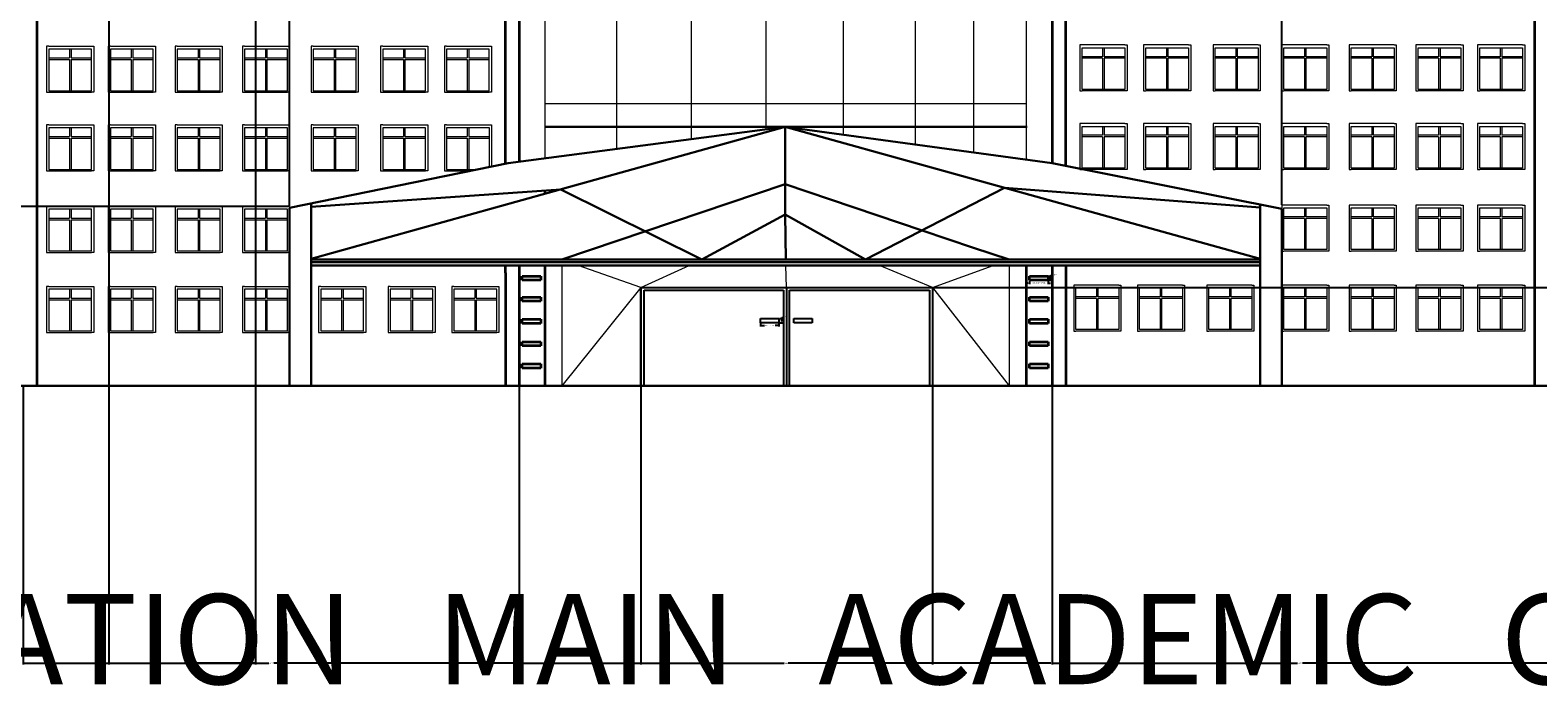
# Model space of a CAD drawing. Units: inches. Extents: x -279 to 364, y -385 to 335.
# Tile 6 of 9: x -60 to 168, y -66 to 34. Entities that reach past the tile are written whole.
import ezdxf

# ---------------------------------------------------------------- set-up
doc = ezdxf.new("R2010")
doc.units = ezdxf.units.IN
doc.header["$MEASUREMENT"] = 0
for name, color, linetype, lineweight in [('A-ANNO-DIMS', 2, 'Continuous', 18), ('A-ANNO-TEXT', 7, 'Continuous', 25), ('A-DOOR', 3, 'Continuous', 25), ('A-GLAZ', 4, 'Continuous', 18), ('A-GLAZ-CURT', 4, 'Continuous', 18), ('A-ROOF-CNPY', 7, 'Continuous', 30), ('A-WALL', 7, 'Continuous', 35), ('C-TOPO', 32, 'Continuous', 30)]:
    doc.layers.add(name, color=color, linetype=linetype, lineweight=lineweight)
doc.styles.get("Standard").update_dxf_attribs({"font": 'arial.ttf'})
doc.dimstyles.get("Standard").update_dxf_attribs({"dimtxt": 0.18, "dimasz": 0.18, "dimexe": 0.18, "dimexo": 0.0625, "dimgap": 0.09, "dimtad": 0, "dimtih": 1, "dimtoh": 1, "dimdec": 4, "dimzin": 0, "dimdsep": 46, "dimtxsty": 'Standard', "dimcen": 0.09, "dimadec": 0, "dimazin": 0, "dimtfac": 1, "dimtdec": 4, "dimtofl": 0, "dimtmove": 0, "dimatfit": 3, "dimfxl": 1, "dimtolj": 1, "dimtzin": 0, "dimarcsym": 0})

# ---------------------------------------------------------------- blocks, each defined once
blk = doc.blocks.new('WIN-TRANSOM-TWIN')
for p, q in [((0.32, 6.97), (0, 6.97)), ((0, 6.97), (0, 0)), ((0.32, 6.97), (6.81, 6.97)), ((6.81, 6.97), (7.13, 6.97)), ((7.13, 6.97), (7.13, 0)), ((0.32, 6.53), (0.32, 0.22)), ((6.81, 6.53), (0.32, 6.53)), ((0.32, 6.53), (0.32, 6.53)), ((0.32, 5.19), (3.48, 5.19)), ((0.32, 4.95), (3.48, 4.95)), ((3.48, 6.53), (3.48, 5.19)), ((3.48, 4.95), (3.48, 0.22)), ((3.69, 6.53), (3.69, 5.19)), ((3.69, 5.19), (6.81, 5.19)), ((3.69, 4.95), (3.69, 0.22)), ((3.69, 4.95), (6.81, 4.95)), ((6.81, 0.22), (6.81, 6.53)), ((0, 0), (0.32, 0)), ((0.32, 0.22), (6.81, 0.22)), ((0.32, 0), (6.81, 0)), ((7.13, 0), (6.81, 0))]:
    blk.add_line(p, q)
blk = doc.blocks.new('PULL-FRONT')
for p, q in [((0, 0.62), (2.81, 0.62)), ((0, 0), (0, 0.62)), ((2.81, 0), (0, 0)), ((2.81, 0.62), (2.81, 0))]:
    blk.add_line(p, q)
blk = doc.blocks.new('PIER-INSET')
for p, q in [((0, 0.62), (2.81, 0.62)), ((0, 0), (0, 0.62)), ((2.81, 0.62), (2.81, 0)), ((2.81, 0), (0, 0))]:
    blk.add_line(p, q)
blk = doc.blocks.new('*D62')
at = {"layer": 'A-ANNO-DIMS', "color": 0, "lineweight": -2, "transparency": 16777216}
for p, q in [((90.63, -4.54), (90.45, -4.54)), ((90.81, -4.18), (90.81, -4.72)), ((93.61, -4.18), (93.61, -4.72)), ((93.79, -4.54), (93.97, -4.54))]:
    blk.add_line(p, q, dxfattribs=at)
at = {"layer": 'A-ANNO-DIMS', "color": 0, "transparency": 16777216}
for points in [[(90.63, -4.51), (90.63, -4.57), (90.81, -4.54)], [(93.79, -4.51), (93.79, -4.57), (93.61, -4.54)]]:
    blk.add_solid(points, dxfattribs=at)
at = {"layer": 'Defpoints', "color": 0, "transparency": 16777216}
for p in [(90.81, -4.12), (93.61, -4.12), (93.61, -4.54)]:
    blk.add_point(p, dxfattribs=at)
at = {"layer": 'A-ANNO-DIMS', "color": 0, "transparency": 16777216, "insert": (92.21, -4.54), "char_height": 0.18, "attachment_point": 5}
blk.add_mtext('\\A1;PIER INSET 3 TYP.', dxfattribs=at)
blk = doc.blocks.new('*D63')
at = {"layer": 'A-ANNO-DIMS', "color": 0, "lineweight": -2, "transparency": 16777216}
for p, q in [((93.68, -3.5), (94.22, -3.5)), ((93.68, -4.12), (94.22, -4.12)), ((94.04, -3.5), (94.04, -3.32)), ((94.04, -3.32), (94.22, -3.32)), ((94.04, -3.94), (94.04, -3.68))]:
    blk.add_line(p, q, dxfattribs=at)
at = {"layer": 'A-ANNO-DIMS', "color": 0, "transparency": 16777216}
for points in [[(94.01, -3.68), (94.07, -3.68), (94.04, -3.5)], [(94.01, -3.94), (94.07, -3.94), (94.04, -4.12)]]:
    blk.add_solid(points, dxfattribs=at)
at = {"layer": 'Defpoints', "color": 0, "transparency": 16777216}
for p in [(93.61, -3.5), (93.61, -4.12), (94.04, -3.5)]:
    blk.add_point(p, dxfattribs=at)
at = {"layer": 'A-ANNO-DIMS', "color": 0, "transparency": 16777216, "insert": (94.67, -3.32), "char_height": 0.18, "attachment_point": 5}
blk.add_mtext('\\A1;1 TYP.', dxfattribs=at)
blk = doc.blocks.new('*D72')
at = {"layer": 'A-ANNO-DIMS', "color": 0, "lineweight": -2, "transparency": 16777216}
for p, q in [((50.08, -10.6), (50.08, -11.14)), ((50.26, -10.96), (50.68, -10.96)), ((52.71, -10.96), (52.29, -10.96)), ((52.89, -10.6), (52.89, -11.14))]:
    blk.add_line(p, q, dxfattribs=at)
at = {"layer": 'A-ANNO-DIMS', "color": 0, "transparency": 16777216}
for points in [[(50.26, -10.93), (50.26, -10.99), (50.08, -10.96)], [(52.71, -10.93), (52.71, -10.99), (52.89, -10.96)]]:
    blk.add_solid(points, dxfattribs=at)
at = {"layer": 'Defpoints', "color": 0, "transparency": 16777216}
for p in [(50.08, -10.54), (52.89, -10.54), (52.89, -10.96)]:
    blk.add_point(p, dxfattribs=at)
at = {"layer": 'A-ANNO-DIMS', "color": 0, "transparency": 16777216, "insert": (51.49, -10.96), "char_height": 0.18, "attachment_point": 5}
blk.add_mtext('\\A1;PULL 3 TYP.', dxfattribs=at)
blk = doc.blocks.new('*D73')
at = {"layer": 'A-ANNO-DIMS', "color": 0, "lineweight": -2, "transparency": 16777216}
for p, q in [((52.95, -9.92), (53.49, -9.92)), ((52.95, -10.54), (53.49, -10.54)), ((53.31, -9.92), (53.31, -9.74)), ((53.31, -9.74), (53.49, -9.74)), ((53.31, -10.36), (53.31, -10.1))]:
    blk.add_line(p, q, dxfattribs=at)
at = {"layer": 'A-ANNO-DIMS', "color": 0, "transparency": 16777216}
for points in [[(53.28, -10.1), (53.34, -10.1), (53.31, -9.92)], [(53.28, -10.36), (53.34, -10.36), (53.31, -10.54)]]:
    blk.add_solid(points, dxfattribs=at)
at = {"layer": 'Defpoints', "color": 0, "transparency": 16777216}
for p in [(52.89, -9.92), (52.89, -10.54), (53.31, -9.92)]:
    blk.add_point(p, dxfattribs=at)
at = {"layer": 'A-ANNO-DIMS', "color": 0, "transparency": 16777216, "insert": (53.94, -9.74), "char_height": 0.18, "attachment_point": 5}
blk.add_mtext('\\A1;1 TYP.', dxfattribs=at)
blk = doc.blocks.new('*D75')
at = {"layer": 'A-ANNO-DIMS', "color": 0, "lineweight": -2, "transparency": 16777216}
for p, q in [((53.76, 188.99), (-212.62, 188.99)), ((-212.44, 188.81), (-212.44, 84.64)), ((-212.44, -19.9), (-212.44, 84.27)), ((-133.86, -20.08), (-212.62, -20.08))]:
    blk.add_line(p, q, dxfattribs=at)
at = {"layer": 'A-ANNO-DIMS', "color": 0, "transparency": 16777216}
for points in [[(-212.47, 188.81), (-212.41, 188.81), (-212.44, 188.99)], [(-212.47, -19.9), (-212.41, -19.9), (-212.44, -20.08)]]:
    blk.add_solid(points, dxfattribs=at)
at = {"layer": 'Defpoints', "color": 0, "transparency": 16777216}
for p in [(-212.44, 188.99), (53.82, 188.99), (-133.8, -20.08)]:
    blk.add_point(p, dxfattribs=at)
at = {"layer": 'A-ANNO-DIMS', "color": 0, "transparency": 16777216, "insert": (-212.44, 84.45), "char_height": 0.18, "attachment_point": 5}
blk.add_mtext('\\A1;209.07', dxfattribs=at)
blk = doc.blocks.new('*D76')
at = {"layer": 'A-ANNO-DIMS', "color": 0, "lineweight": -2, "transparency": 16777216}
for p, q in [((17.12, 147.82), (-212.62, 147.82)), ((-212.44, 147.64), (-212.44, 64.05)), ((-212.44, -19.9), (-212.44, 63.68)), ((17.4, -20.08), (-212.62, -20.08))]:
    blk.add_line(p, q, dxfattribs=at)
at = {"layer": 'A-ANNO-DIMS', "color": 0, "transparency": 16777216}
for points in [[(-212.47, 147.64), (-212.41, 147.64), (-212.44, 147.82)], [(-212.47, -19.9), (-212.41, -19.9), (-212.44, -20.08)]]:
    blk.add_solid(points, dxfattribs=at)
at = {"layer": 'Defpoints', "color": 0, "transparency": 16777216}
for p in [(-212.44, 147.82), (17.19, 147.82), (17.46, -20.08)]:
    blk.add_point(p, dxfattribs=at)
at = {"layer": 'A-ANNO-DIMS', "color": 0, "transparency": 16777216, "insert": (-212.44, 63.87), "char_height": 0.18, "attachment_point": 5}
blk.add_mtext('\\A1;167.9', dxfattribs=at)
blk = doc.blocks.new('*D78')
at = {"layer": 'A-ANNO-DIMS', "color": 0, "lineweight": -2, "transparency": 16777216}
for p, q in [((-61.49, -20.14), (-61.49, -62.3)), ((13.58, -20.14), (13.58, -62.3)), ((-61.31, -62.12), (-24.34, -62.12)), ((13.4, -62.12), (-23.56, -62.12))]:
    blk.add_line(p, q, dxfattribs=at)
at = {"layer": 'A-ANNO-DIMS', "color": 0, "transparency": 16777216}
for points in [[(-61.31, -62.09), (-61.31, -62.15), (-61.49, -62.12)], [(13.4, -62.09), (13.4, -62.15), (13.58, -62.12)]]:
    blk.add_solid(points, dxfattribs=at)
at = {"layer": 'Defpoints', "color": 0, "transparency": 16777216}
for p in [(-61.49, -20.08), (13.58, -20.08), (13.58, -62.12)]:
    blk.add_point(p, dxfattribs=at)
at = {"layer": 'A-ANNO-DIMS', "color": 0, "transparency": 16777216, "insert": (-23.95, -62.12), "char_height": 0.18, "attachment_point": 5}
blk.add_mtext('\\A1;75.07', dxfattribs=at)
blk = doc.blocks.new('*D79')
at = {"layer": 'A-ANNO-DIMS', "color": 0, "lineweight": -2, "transparency": 16777216}
for p, q in [((13.58, -20.14), (13.58, -62.3)), ((94.22, -19.95), (94.22, -62.3)), ((13.76, -62.12), (53.51, -62.12)), ((94.04, -62.12), (54.3, -62.12))]:
    blk.add_line(p, q, dxfattribs=at)
at = {"layer": 'A-ANNO-DIMS', "color": 0, "transparency": 16777216}
for points in [[(13.76, -62.09), (13.76, -62.15), (13.58, -62.12)], [(94.04, -62.09), (94.04, -62.15), (94.22, -62.12)]]:
    blk.add_solid(points, dxfattribs=at)
at = {"layer": 'Defpoints', "color": 0, "transparency": 16777216}
for p in [(13.58, -20.08), (94.22, -19.89), (94.22, -62.12)]:
    blk.add_point(p, dxfattribs=at)
at = {"layer": 'A-ANNO-DIMS', "color": 0, "transparency": 16777216, "insert": (53.9, -62.12), "char_height": 0.18, "attachment_point": 5}
blk.add_mtext('\\A1;80.64', dxfattribs=at)
blk = doc.blocks.new('*D80')
at = {"layer": 'A-ANNO-DIMS', "color": 0, "lineweight": -2, "transparency": 16777216}
for p, q in [((94.22, -19.95), (94.22, -62.3)), ((169.29, -19.95), (169.29, -62.3)), ((94.4, -62.12), (131.36, -62.12)), ((169.11, -62.12), (132.15, -62.12))]:
    blk.add_line(p, q, dxfattribs=at)
at = {"layer": 'A-ANNO-DIMS', "color": 0, "transparency": 16777216}
for points in [[(94.4, -62.09), (94.4, -62.15), (94.22, -62.12)], [(169.11, -62.09), (169.11, -62.15), (169.29, -62.12)]]:
    blk.add_solid(points, dxfattribs=at)
at = {"layer": 'Defpoints', "color": 0, "transparency": 16777216}
for p in [(94.22, -19.89), (169.29, -19.89), (169.29, -62.12)]:
    blk.add_point(p, dxfattribs=at)
at = {"layer": 'A-ANNO-DIMS', "color": 0, "transparency": 16777216, "insert": (131.76, -62.12), "char_height": 0.18, "attachment_point": 5}
blk.add_mtext('\\A1;75.07', dxfattribs=at)
blk = doc.blocks.new('*D92')
at = {"layer": 'A-ANNO-DIMS', "color": 0, "lineweight": -2, "transparency": 16777216}
for p, q in [((-48.53, 57.83), (-48.53, -62.3)), ((-26.33, 57.83), (-26.33, -62.3)), ((-48.35, -62.12), (-37.75, -62.12)), ((-26.51, -62.12), (-37.11, -62.12))]:
    blk.add_line(p, q, dxfattribs=at)
at = {"layer": 'A-ANNO-DIMS', "color": 0, "transparency": 16777216}
for points in [[(-48.35, -62.09), (-48.35, -62.15), (-48.53, -62.12)], [(-26.51, -62.09), (-26.51, -62.15), (-26.33, -62.12)]]:
    blk.add_solid(points, dxfattribs=at)
at = {"layer": 'Defpoints', "color": 0, "transparency": 16777216}
for p in [(-48.53, 57.89), (-26.33, 57.89), (-26.33, -62.12)]:
    blk.add_point(p, dxfattribs=at)
at = {"layer": 'A-ANNO-DIMS', "color": 0, "transparency": 16777216, "insert": (-37.43, -62.12), "char_height": 0.18, "attachment_point": 5}
blk.add_mtext('\\A1;22.2', dxfattribs=at)
blk = doc.blocks.new('*D93')
at = {"layer": 'A-ANNO-DIMS', "color": 0, "lineweight": -2, "transparency": 16777216}
for p, q in [((-21.19, 7.14), (-21.19, 213.67)), ((-21.01, 213.49), (53.45, 213.49)), ((128.81, 213.49), (54.36, 213.49)), ((128.99, 7.33), (128.99, 213.67))]:
    blk.add_line(p, q, dxfattribs=at)
at = {"layer": 'A-ANNO-DIMS', "color": 0, "transparency": 16777216}
for points in [[(-21.01, 213.52), (-21.01, 213.46), (-21.19, 213.49)], [(128.81, 213.52), (128.81, 213.46), (128.99, 213.49)]]:
    blk.add_solid(points, dxfattribs=at)
at = {"layer": 'Defpoints', "color": 0, "transparency": 16777216}
for p in [(128.99, 213.49), (-21.19, 7.08), (128.99, 7.27)]:
    blk.add_point(p, dxfattribs=at)
at = {"layer": 'A-ANNO-DIMS', "color": 0, "transparency": 16777216, "insert": (53.9, 213.49), "char_height": 0.18, "attachment_point": 5}
blk.add_mtext('\\A1;150.18', dxfattribs=at)
blk = doc.blocks.new('*D94')
at = {"layer": 'A-ANNO-DIMS', "color": 0, "lineweight": -2, "transparency": 16777216}
for p, q in [((-21.25, 7.08), (-212.62, 7.08)), ((-212.44, 6.9), (-212.44, -6.32)), ((-212.44, -19.9), (-212.44, -6.68)), ((-21.25, -20.08), (-212.62, -20.08))]:
    blk.add_line(p, q, dxfattribs=at)
at = {"layer": 'A-ANNO-DIMS', "color": 0, "transparency": 16777216}
for points in [[(-212.47, 6.9), (-212.41, 6.9), (-212.44, 7.08)], [(-212.47, -19.9), (-212.41, -19.9), (-212.44, -20.08)]]:
    blk.add_solid(points, dxfattribs=at)
at = {"layer": 'Defpoints', "color": 0, "transparency": 16777216}
for p in [(-212.44, 7.08), (-21.19, 7.08), (-21.19, -20.08)]:
    blk.add_point(p, dxfattribs=at)
at = {"layer": 'A-ANNO-DIMS', "color": 0, "transparency": 16777216, "insert": (-212.44, -6.5), "char_height": 0.18, "attachment_point": 5}
blk.add_mtext('\\A1;27.16', dxfattribs=at)
blk = doc.blocks.new('*D95')
at = {"layer": 'A-ANNO-DIMS', "color": 0, "lineweight": -2, "transparency": 16777216}
for p, q in [((32, -5.29), (32, -62.3)), ((76.12, -5.29), (76.12, -62.3)), ((32.18, -62.12), (53.66, -62.12)), ((75.94, -62.12), (54.45, -62.12))]:
    blk.add_line(p, q, dxfattribs=at)
at = {"layer": 'A-ANNO-DIMS', "color": 0, "transparency": 16777216}
for points in [[(32.18, -62.09), (32.18, -62.15), (32, -62.12)], [(75.94, -62.09), (75.94, -62.15), (76.12, -62.12)]]:
    blk.add_solid(points, dxfattribs=at)
at = {"layer": 'Defpoints', "color": 0, "transparency": 16777216}
for p in [(32, -5.23), (76.12, -5.23), (76.12, -62.12)]:
    blk.add_point(p, dxfattribs=at)
at = {"layer": 'A-ANNO-DIMS', "color": 0, "transparency": 16777216, "insert": (54.06, -62.12), "char_height": 0.18, "attachment_point": 5}
blk.add_mtext('\\A1;44.12', dxfattribs=at)
blk = doc.blocks.new('*D96')
at = {"layer": 'A-ANNO-DIMS', "color": 0, "lineweight": -2, "transparency": 16777216}
for p, q in [((76.18, -5.23), (323.06, -5.23)), ((322.88, -5.41), (322.88, -12.47)), ((322.88, -19.9), (322.88, -12.84)), ((75.75, -20.08), (323.06, -20.08))]:
    blk.add_line(p, q, dxfattribs=at)
at = {"layer": 'A-ANNO-DIMS', "color": 0, "transparency": 16777216}
for points in [[(322.85, -5.41), (322.91, -5.41), (322.88, -5.23)], [(322.85, -19.9), (322.91, -19.9), (322.88, -20.08)]]:
    blk.add_solid(points, dxfattribs=at)
at = {"layer": 'Defpoints', "color": 0, "transparency": 16777216}
for p in [(76.12, -5.23), (322.88, -5.23), (75.69, -20.08)]:
    blk.add_point(p, dxfattribs=at)
at = {"layer": 'A-ANNO-DIMS', "color": 0, "transparency": 16777216, "insert": (322.88, -12.66), "char_height": 0.18, "attachment_point": 5}
blk.add_mtext('\\A1;14.854', dxfattribs=at)

msp = doc.modelspace()

# ---------------------------------------------------------------- linework, layer by layer
at = {"layer": 'A-DOOR'}
for p, q in [((31.9982, -20.0818), (31.9982, -5.2282)), ((31.9982, -5.2282), (76.1172, -5.2282)), ((32.4653, -20.0818), (32.4653, -5.6279)), ((32.4653, -5.6279), (53.5569, -5.6279)), ((53.5569, -5.6279), (53.5569, -20.0818)), ((54.0034, -5.2282), (54.0034, -20.0818)), ((54.492, -20.0818), (54.492, -5.6279)), ((54.492, -5.6279), (75.6857, -5.6279)), ((75.6857, -5.6279), (75.6857, -20.0818)), ((76.1172, -5.2282), (76.1172, -20.0818)), ((31.9982, -20.0818), (31.9982, -20.0818)), ((31.9982, -20.0818), (31.9982, -20.0818))]:
    msp.add_line(p, q, dxfattribs=at)
at = {"layer": 'A-GLAZ'}
for p, q in [((2.5546, 19.4258), (2.2361, 19.4258)), ((2.2361, 19.4258), (2.2361, 12.4606)), ((2.5546, 19.4258), (9.0497, 19.4258)), ((2.5546, 18.9905), (2.5546, 12.6834)), ((9.0497, 18.9905), (2.5546, 18.9905)), ((2.5546, 18.9905), (2.5546, 18.9905)), ((5.7119, 18.9905), (5.7119, 17.6537)), ((5.9241, 18.9905), (5.9241, 17.6537)), ((9.0497, 19.4258), (9.369, 19.4258)), ((9.0497, 13.0254), (9.0497, 18.9905)), ((9.369, 19.4258), (9.369, 13.0908)), ((2.5546, 17.6537), (5.7119, 17.6537)), ((2.5546, 17.4137), (5.7119, 17.4137)), ((5.7119, 17.4137), (5.7119, 12.6834)), ((5.9241, 17.6537), (9.0497, 17.6537)), ((5.9241, 17.4137), (9.0497, 17.4137)), ((5.9241, 17.4137), (5.9241, 12.6834)), ((2.2361, 12.4606), (2.5546, 12.4606)), ((2.5546, 12.6834), (7.3795, 12.6834)), ((2.5546, 12.4606), (6.2918, 12.4606))]:
    msp.add_line(p, q, dxfattribs=at)
at = {"layer": 'A-GLAZ-CURT'}
for p, q in [((17.4585, 126.6636), (17.4585, 14.3396)), ((28.3065, 126.6636), (28.3065, 15.7643)), ((39.6009, 126.6636), (39.6009, 17.2476)), ((50.8952, 126.6636), (50.8952, 18.7309)), ((62.5929, 126.6636), (62.5929, 17.9201)), ((73.4839, 126.6636), (73.4839, 16.4361)), ((82.358, 126.6636), (82.358, 15.227)), ((90.3118, 68.1077), (90.3118, 14.1432)), ((17.4585, 22.6364), (90.3118, 22.6364)), ((20.0417, -1.858), (20.0417, -20.0818)), ((31.9982, -5.2282), (22.5029, -1.858)), ((31.9982, -5.2282), (39.3135, -1.858)), ((54.0034, -5.2282), (53.9482, -1.858)), ((76.1172, -5.2282), (68.0839, -1.858)), ((76.1172, -5.2282), (85.3313, -1.858)), ((87.7196, -1.858), (87.7196, -20.0818)), ((31.9982, -5.2282), (20.0417, -20.0818)), ((76.1172, -5.2282), (87.7196, -20.0818))]:
    msp.add_line(p, q, dxfattribs=at)
at = {"layer": 'A-ROOF-CNPY'}
for p, q in [((53.8218, 19.1153), (-17.9142, -0.8832)), ((11.9057, 13.6104), (53.8218, 19.1153)), ((17.4585, 19.1153), (90.4567, 19.1153)), ((53.8218, 19.1153), (125.7192, -0.8853)), ((94.2224, 13.6104), (53.8218, 19.1153)), ((53.8218, 10.4395), (53.8218, 19.1153)), ((94.2202, 19.1153), (94.2224, 19.1153)), ((94.2224, 13.6104), (94.2224, 19.1153)), ((-21.1877, 6.8325), (11.9057, 13.6104)), ((128.9927, 6.6954), (94.2224, 13.6104)), ((19.8617, 9.6479), (-17.9142, 7.0292)), ((17.4585, 9.4813), (17.4585, 8.9779)), ((41.2097, -0.9844), (19.8617, 9.6479)), ((20.0417, -0.9844), (53.8218, 10.4395)), ((53.8218, 10.4395), (74.5704, 3.447)), ((53.8218, 10.4395), (53.8218, 5.8637)), ((66.0016, -0.9844), (87.0132, 9.882)), ((87.0132, 9.882), (125.7192, 6.9187)), ((-17.9142, 7.0292), (-17.9142, 7.5029)), ((-17.9142, -0.9844), (-17.9142, 7.0292)), ((90.3118, 8.9644), (90.3118, 8.9602)), ((125.7192, -0.9844), (125.7192, 7.3464)), ((-21.1877, 6.8023), (-21.1877, -20.0818)), ((53.8218, 5.8637), (41.2097, -0.9844)), ((53.8218, 5.8637), (66.0016, -0.9844)), ((53.9339, -0.9844), (53.8218, 5.8637)), ((128.9927, 6.6681), (128.9927, -20.0818)), ((74.5704, 3.447), (82.358, 0.8225)), ((82.358, 0.8225), (87.7196, -0.9844)), ((-17.9142, -0.9844), (-17.9142, -0.8832)), ((-17.9142, -0.9844), (125.7192, -0.9844)), ((-17.9142, -0.9844), (-17.9142, -1.858)), ((-17.9142, -1.3908), (125.7192, -1.3908)), ((-17.9142, -1.858), (125.7192, -1.858)), ((-17.9142, -20.0818), (-17.9142, -1.858)), ((125.7192, -0.9844), (125.7192, -1.858)), ((125.7192, -20.0818), (125.7192, -1.858)), ((-17.9142, -12.0084), (-17.9142, -20.0818)), ((125.7192, -11.8149), (125.7192, -20.0818))]:
    msp.add_line(p, q, dxfattribs=at)
at = {"layer": 'A-WALL'}
for p, q in [((13.5848, 118.4445), (13.5848, 13.8309)), ((94.2202, 118.6379), (94.2202, 13.6107)), ((-59.4257, 115.9949), (-59.4257, -2.9883)), ((11.51, 13.5293), (11.51, 115.9949)), ((96.295, 13.1982), (96.295, 116.1883)), ((167.2307, 116.1883), (167.2307, -2.7949)), ((11.51, -2.9883), (11.51, -1.858)), ((13.5848, -1.858), (13.5848, -2.9883)), ((17.4585, -1.858), (17.4585, -20.0818)), ((90.3118, -1.858), (90.3118, -20.0818)), ((94.2202, -1.858), (94.2202, -2.7949)), ((96.295, -1.858), (96.295, -20.0818)), ((-59.4257, -2.9883), (-59.4257, -20.0818)), ((11.51, -2.9883), (11.51, -20.0818)), ((13.5848, -2.9883), (13.5848, -20.0818)), ((94.2202, -2.7949), (94.2202, -19.8884)), ((167.2307, -2.7949), (167.2307, -19.8884))]:
    msp.add_line(p, q, dxfattribs=at)
at = {"layer": 'C-TOPO'}
for p in [(-133.7987, -20.0818), (31.9982, -20.0818)]:
    msp.add_line(p, (198.4631, -20.0818), dxfattribs=at)

# ---------------------------------------------------------------- block references
at = {"layer": 'A-DOOR'}
for p in [(50.08, -10.536), (55.1207, -10.536)]:
    msp.add_blockref('PULL-FRONT', p, dxfattribs=at)
at = {"layer": 'A-GLAZ'}
for p in [(-57.96, 24.3586), (-48.6248, 24.3586), (-38.5023, 24.3586), (-28.321, 24.3586), (-17.9147, 24.3586), (-7.4138, 24.3586), (2.2357, 24.3586), (-57.96, 12.4603), (-48.6248, 12.4603), (-38.5023, 12.4603), (-28.321, 12.4603), (-17.9147, 12.4603), (-7.4138, 12.4603), (-57.96, 0.1107), (-48.6248, 0.1107), (-38.5023, 0.1107), (-28.321, 0.1107), (-57.96, -12.0086), (-48.6248, -12.0086), (-38.5023, -12.0086), (-28.321, -12.0086), (-16.7917, -12.0086), (-6.2908, -12.0086), (3.3587, -12.0086)]:
    msp.add_blockref('WIN-TRANSOM-TWIN', p, dxfattribs=at)
at = {"layer": 'A-GLAZ', "extrusion": (0, 0, -1), "zscale": -1}
for p in [(-105.5693, 24.552), (-115.2187, 24.552), (-125.7196, 24.552), (-136.1259, 24.552), (-146.3073, 24.552), (-156.4298, 24.552), (-165.765, 24.552), (-105.5693, 12.6537), (-115.2187, 12.6537), (-125.7196, 12.6537), (-136.1259, 12.6537), (-146.3073, 12.6537), (-156.4298, 12.6537), (-165.765, 12.6537), (-136.1259, 0.3042), (-146.3073, 0.3042), (-156.4298, 0.3042), (-165.765, 0.3042), (-104.6303, -11.8152), (-114.2797, -11.8152), (-124.7806, -11.8152), (-136.1259, -11.8152), (-146.3073, -11.8152), (-156.4298, -11.8152), (-165.765, -11.8152)]:
    msp.add_blockref('WIN-TRANSOM-TWIN', p, dxfattribs=at)
at = {"layer": 'A-WALL'}
for p in [(14.034, -4.119), (90.805, -4.119), (14.034, -7.2932), (90.805, -7.2932), (14.034, -10.6475), (90.805, -10.6475), (14.034, -14.0632), (90.805, -14.0632), (14.034, -17.4092), (90.805, -17.4092)]:
    msp.add_blockref('PIER-INSET', p, dxfattribs=at)

# ---------------------------------------------------------------- texts
at = {"layer": 'A-ANNO-TEXT'}
msp.add_text('FRONT   ELEVATION   MAIN   ACADEMIC   COMPLEX', height=13.648689, dxfattribs=at).set_placement((-182.5362, -65.301))

# ---------------------------------------------------------------- dimensions: what is measured, and where the dimension line sits
at = {"layer": 'A-ANNO-DIMS'}
for base, p1, p2, override, picture, middle in [((128.9927, 213.4896), (-21.1877, 7.0763), (128.9927, 7.2697), {"dimdec": 2, "dimlfac": 1, "dimrnd": 0, "dimzin": 0, "dimdsep": 46, "dimlunit": 2}, '*D93', (53.9025, 213.4896)), ((-26.3293, -62.1247), (-48.5304, 57.8883), (-26.3293, 57.8883), {"dimdec": 1, "dimlfac": 1, "dimrnd": 0, "dimzin": 0, "dimdsep": 46, "dimlunit": 2}, '*D92', (-37.4299, -62.1247)), ((76.1172, -62.1247), (31.9982, -5.2282), (76.1172, -5.2282), {"dimdec": 2, "dimlfac": 1, "dimrnd": 0, "dimzin": 0, "dimdsep": 46, "dimlunit": 2}, '*D95', (54.0577, -62.1247)), ((13.5848, -62.1247), (-61.4888, -20.0818), (13.5848, -20.0818), {"dimdec": 2, "dimlfac": 1, "dimrnd": 0, "dimzin": 0, "dimdsep": 46, "dimlunit": 2}, '*D78', (-23.952, -62.1247)), ((94.2202, -62.1247), (13.5848, -20.0818), (94.2202, -19.8884), {"dimdec": 2, "dimlfac": 1, "dimrnd": 0, "dimzin": 0, "dimdsep": 46, "dimlunit": 2}, '*D79', (53.9025, -62.1247)), ((169.2937, -62.1247), (94.2202, -19.8884), (169.2937, -19.8884), {"dimdec": 2, "dimlfac": 1, "dimrnd": 0, "dimzin": 0, "dimdsep": 46, "dimlunit": 2}, '*D80', (131.757, -62.1247))]:
    dim = msp.add_linear_dim(base=base, p1=p1, p2=p2, dimstyle='Standard', override=override, dxfattribs=at)
    dim.commit()
    dim.dimension.update_dxf_attribs({"geometry": picture, "text_midpoint": middle})
for base, p1, p2, override, picture, middle in [((-212.4386, 188.9896), (-133.7987, -20.0818), (53.8218, 188.9896), {"dimdec": 2, "dimlfac": 1, "dimrnd": 0, "dimzin": 0, "dimdsep": 46, "dimlunit": 2}, '*D75', (-212.4386, 84.4539)), ((-212.4386, 147.8151), (17.4585, -20.0818), (17.1869, 147.8151), {"dimdec": 1, "dimlfac": 1, "dimrnd": 0, "dimzin": 0, "dimdsep": 46, "dimlunit": 2}, '*D76', (-212.4386, 63.8666)), ((-212.4386, 7.0763), (-21.1877, -20.0818), (-21.1877, 7.0763), {"dimdec": 2, "dimlfac": 1, "dimrnd": 0, "dimzin": 0, "dimdsep": 46, "dimlunit": 2}, '*D94', (-212.4386, -6.5028)), ((322.8779, -5.2282), (75.6857, -20.0818), (76.1172, -5.2282), {"dimdec": 3, "dimlfac": 1, "dimrnd": 0, "dimzin": 0, "dimdsep": 46, "dimlunit": 2}, '*D96', (322.8779, -12.655))]:
    dim = msp.add_linear_dim(base=base, p1=p1, p2=p2, angle=90, dimstyle='Standard', override=override, dxfattribs=at)
    dim.commit()
    dim.dimension.update_dxf_attribs({"geometry": picture, "text_midpoint": middle})
for base, p1, p2, text, picture, middle in [((93.6147, -4.5407), (90.8051, -4.1193), (93.6147, -4.1193), 'PIER INSET <> TYP.', '*D62', (92.2099, -4.5407)), ((52.89, -10.9573), (50.0804, -10.5359), (52.89, -10.5359), 'PULL <> TYP.', '*D72', (51.4852, -10.9573))]:
    dim = msp.add_linear_dim(base=base, p1=p1, p2=p2, text=text, dimstyle='Standard', override={"dimdec": 0, "dimlfac": 1, "dimrnd": 0, "dimzin": 0, "dimdsep": 46, "dimlunit": 2}, dxfattribs=at)
    dim.commit()
    dim.dimension.update_dxf_attribs({"geometry": picture, "text_midpoint": middle})
for base, p1, p2, picture, middle in [((94.0361, -3.5003), (93.6147, -4.1193), (93.6147, -3.5003), '*D63', (94.6658, -3.3203)), ((53.3114, -9.9169), (52.89, -10.5359), (52.89, -9.9169), '*D73', (53.9411, -9.7369))]:
    dim = msp.add_linear_dim(base=base, p1=p1, p2=p2, angle=90, text='<> TYP.', dimstyle='Standard', override={"dimdec": 0, "dimlfac": 1, "dimrnd": 0, "dimzin": 0, "dimdsep": 46, "dimlunit": 2}, dxfattribs=at)
    dim.commit()
    dim.dimension.update_dxf_attribs({"geometry": picture, "text_midpoint": middle})

doc.saveas('drawing.dxf')
